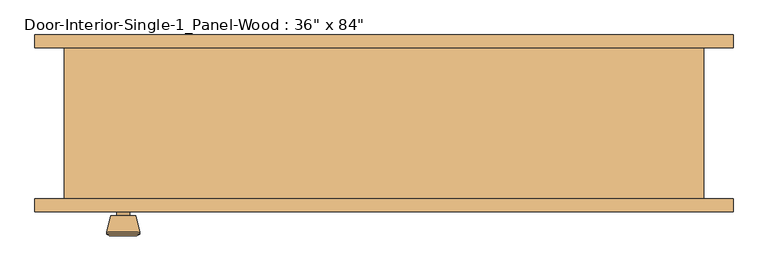
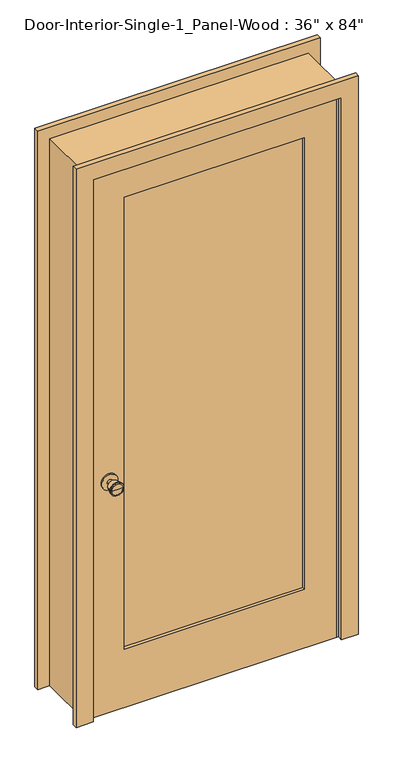
"""IFC4 building model written with IfcOpenShell, lengths in millimetres: door geometry."""

from ifc_helpers import new_model, si_unit, point, frame, frame_2d, origin, place, context, project, spatial, polyline, circle_curve, trimmed, segment, composite_curve, outline, extrude, faceted_brep, source, transform, mapped, element, save
from ifc_brep_helpers import plane_surface, cylinder_surface, revolved_surface, advanced_brep


def door_868ee8a9(model_context):
    return source(origin(), model_context, "Body", "SolidModel", [
        advanced_brep(
        [(-393.7, -70.2, 914.4), (-403.7, -70.2, 914.4), (-383.7, -70.2, 914.4), (-373.2241324, -21.2, 914.4), (-414.1758676, -21.2, 914.4), (-393.7, -21.2, 914.4), (-368.7, -23.0278681, 914.4), (-418.7, -23.0278681, 914.4), (-368.7, -26.4915463, 914.4), (-418.7, -26.4915463, 914.4), (-375.063764, -51.2, 914.4), (-412.336236, -51.2, 914.4), (-383.7, -51.2, 914.4), (-403.7, -51.2, 914.4)],
        [
            (0, 1),
            (1, 2, circle_curve(frame((-393.7, -70.2, 914.4), z_axis=(0.0, -1.0, 0.0), x_axis=(-1.0, 0.0, 0.0)), 10.0)),
            (2, 0),
            (2, 1, circle_curve(frame((-393.7, -70.2, 914.4), z_axis=(0.0, -1.0, 0.0), x_axis=(-1.0, 0.0, 0.0)), 10.0)),
            (3, 4, circle_curve(frame((-393.7, -21.2, 914.4), z_axis=(0.0, 1.0, 0.0), x_axis=(-1.0, 0.0, 0.0)), 20.4758676)),
            (4, 5),
            (5, 3),
            (4, 3, circle_curve(frame((-393.7, -21.2, 914.4), z_axis=(0.0, 1.0, 0.0), x_axis=(-1.0, 0.0, 0.0)), 20.4758676)),
            (6, 7, circle_curve(frame((-393.7, -23.0278681, 914.4), z_axis=(0.0, 1.0, 0.0), x_axis=(-1.0, 0.0, 0.0)), 25.0)),
            (7, 4),
            (3, 6),
            (7, 6, circle_curve(frame((-393.7, -23.0278681, 914.4), z_axis=(0.0, 1.0, 0.0), x_axis=(-1.0, 0.0, 0.0)), 25.0)),
            (8, 9, circle_curve(frame((-393.7, -26.4915463, 914.4), z_axis=(0.0, 1.0, 0.0), x_axis=(-1.0, 0.0, 0.0)), 25.0)),
            (9, 7),
            (6, 8),
            (9, 8, circle_curve(frame((-393.7, -26.4915463, 914.4), z_axis=(0.0, 1.0, 0.0), x_axis=(-1.0, 0.0, 0.0)), 25.0)),
            (10, 11, circle_curve(frame((-393.7, -51.2, 914.4), z_axis=(0.0, 1.0, 0.0), x_axis=(-1.0, 0.0, 0.0)), 18.636236)),
            (11, 9),
            (8, 10),
            (11, 10, circle_curve(frame((-393.7, -51.2, 914.4), z_axis=(0.0, 1.0, 0.0), x_axis=(-1.0, 0.0, 0.0)), 18.636236)),
            (12, 13, circle_curve(frame((-393.7, -51.2, 914.4), z_axis=(0.0, 1.0, 0.0), x_axis=(-1.0, 0.0, 0.0)), 10.0)),
            (13, 11),
            (10, 12),
            (13, 12, circle_curve(frame((-393.7, -51.2, 914.4), z_axis=(0.0, 1.0, 0.0), x_axis=(-1.0, 0.0, 0.0)), 10.0)),
            (1, 13),
            (12, 2),
        ],
        [
            plane_surface(frame((-393.7, -70.2, 914.4), z_axis=(0.0, -1.0, 0.0), x_axis=(-1.0, 0.0, 0.0))),
            plane_surface(frame((-393.7, -21.2, 914.4), z_axis=(0.0, 1.0, 0.0), x_axis=(-1.0, 0.0, 0.0))),
            revolved_surface(polyline([(-414.1758676, -21.2, 914.4), (-418.7, -23.0278681, 914.4)]), (-393.7, -70.2, 914.4), (0.0, -1.0, 0.0)),
            cylinder_surface(frame((-393.7, -70.2, 914.4), z_axis=(0.0, -1.0, 0.0), x_axis=(-1.0, 0.0, 0.0)), 25.0),
            revolved_surface(polyline([(-418.7, -26.4915463, 914.4), (-412.336236, -51.2, 914.4)]), (-393.7, -70.2, 914.4), (0.0, -1.0, 0.0)),
            plane_surface(frame((-393.7, -51.2, 914.4), z_axis=(0.0, -1.0, 0.0), x_axis=(-1.0, 0.0, 0.0))),
            cylinder_surface(frame((-393.7, -70.2, 914.4), z_axis=(0.0, -1.0, 0.0), x_axis=(-1.0, 0.0, 0.0)), 10.0),
        ],
        [
            (0, [[1, 2, 3]]),
            (0, [[-3, 4, -1]]),
            (1, [[5, 6, 7]]),
            (1, [[8, -7, -6]]),
            (2, [[9, 10, -5, 11]]),
            (2, [[12, -11, -8, -10]]),
            (3, [[13, 14, -9, 15]]),
            (3, [[16, -15, -12, -14]]),
            (4, [[17, 18, -13, 19]]),
            (4, [[20, -19, -16, -18]]),
            (5, [[21, 22, -17, 23]]),
            (5, [[24, -23, -20, -22]]),
            (6, [[-2, 25, -21, 26]]),
            (6, [[-4, -26, -24, -25]]),
        ],
    ),
        extrude(outline(composite_curve([segment(trimmed(circle_curve(frame_2d((914.4, -393.7)), 30.0), [point((914.4, -423.7))], [point((914.4, -363.7))], False, "CARTESIAN"), True, "CONTINUOUS"), segment(trimmed(circle_curve(frame_2d((914.4, -393.7)), 30.0), [point((914.4, -363.7))], [point((914.4, -423.7))], False, "CARTESIAN"), True, "CONTINUOUS")], self_intersect=False)), frame((0.0, -76.2, 0.0), z_axis=(0.0, 1.0, 0.0), x_axis=(0.0, 0.0, 1.0)), (0.0, 0.0, 1.0), 6.0),
        advanced_brep(
        [(-393.7, -117.125, 914.4), (-383.7, -117.125, 914.4), (-403.7, -117.125, 914.4), (-373.2241324, -166.125, 914.4), (-393.7, -166.125, 914.4), (-414.1758676, -166.125, 914.4), (-368.7, -164.2971319, 914.4), (-418.7, -164.2971319, 914.4), (-368.7, -160.8334537, 914.4), (-418.7, -160.8334537, 914.4), (-375.063764, -136.125, 914.4), (-412.336236, -136.125, 914.4), (-383.7, -136.125, 914.4), (-403.7, -136.125, 914.4)],
        [
            (0, 1),
            (1, 2, circle_curve(frame((-393.7, -117.125, 914.4), z_axis=(0.0, 1.0, 0.0), x_axis=(-1.0, 0.0, 0.0)), 10.0)),
            (2, 0),
            (2, 1, circle_curve(frame((-393.7, -117.125, 914.4), z_axis=(0.0, 1.0, 0.0), x_axis=(-1.0, 0.0, 0.0)), 10.0)),
            (3, 4),
            (4, 5),
            (5, 3, circle_curve(frame((-393.7, -166.125, 914.4), z_axis=(0.0, -1.0, 0.0), x_axis=(-1.0, 0.0, 0.0)), 20.4758676)),
            (3, 5, circle_curve(frame((-393.7, -166.125, 914.4), z_axis=(0.0, -1.0, 0.0), x_axis=(-1.0, 0.0, 0.0)), 20.4758676)),
            (6, 3),
            (5, 7),
            (7, 6, circle_curve(frame((-393.7, -164.2971319, 914.4), z_axis=(0.0, -1.0, 0.0), x_axis=(-1.0, 0.0, 0.0)), 25.0)),
            (6, 7, circle_curve(frame((-393.7, -164.2971319, 914.4), z_axis=(0.0, -1.0, 0.0), x_axis=(-1.0, 0.0, 0.0)), 25.0)),
            (8, 6),
            (7, 9),
            (9, 8, circle_curve(frame((-393.7, -160.8334537, 914.4), z_axis=(0.0, -1.0, 0.0), x_axis=(-1.0, 0.0, 0.0)), 25.0)),
            (8, 9, circle_curve(frame((-393.7, -160.8334537, 914.4), z_axis=(0.0, -1.0, 0.0), x_axis=(-1.0, 0.0, 0.0)), 25.0)),
            (10, 8),
            (9, 11),
            (11, 10, circle_curve(frame((-393.7, -136.125, 914.4), z_axis=(0.0, -1.0, 0.0), x_axis=(-1.0, 0.0, 0.0)), 18.636236)),
            (10, 11, circle_curve(frame((-393.7, -136.125, 914.4), z_axis=(0.0, -1.0, 0.0), x_axis=(-1.0, 0.0, 0.0)), 18.636236)),
            (12, 10),
            (11, 13),
            (13, 12, circle_curve(frame((-393.7, -136.125, 914.4), z_axis=(0.0, -1.0, 0.0), x_axis=(-1.0, 0.0, 0.0)), 10.0)),
            (12, 13, circle_curve(frame((-393.7, -136.125, 914.4), z_axis=(0.0, -1.0, 0.0), x_axis=(-1.0, 0.0, 0.0)), 10.0)),
            (1, 12),
            (13, 2),
        ],
        [
            plane_surface(frame((-393.7, -117.125, 914.4), z_axis=(0.0, 1.0, 0.0), x_axis=(-1.0, 0.0, 0.0))),
            plane_surface(frame((-393.7, -166.125, 914.4), z_axis=(0.0, -1.0, 0.0), x_axis=(-1.0, 0.0, 0.0))),
            revolved_surface(polyline([(-414.1758676, -166.125, 914.4), (-418.7, -164.2971319, 914.4)]), (-393.7, -117.125, 914.4), (0.0, 1.0, 0.0)),
            cylinder_surface(frame((-393.7, -117.125, 914.4), z_axis=(0.0, 1.0, 0.0), x_axis=(-1.0, 0.0, 0.0)), 25.0),
            revolved_surface(polyline([(-418.7, -160.8334537, 914.4), (-412.336236, -136.125, 914.4)]), (-393.7, -117.125, 914.4), (0.0, 1.0, 0.0)),
            plane_surface(frame((-393.7, -136.125, 914.4), z_axis=(0.0, 1.0, 0.0), x_axis=(-1.0, 0.0, 0.0))),
            cylinder_surface(frame((-393.7, -117.125, 914.4), z_axis=(0.0, 1.0, 0.0), x_axis=(-1.0, 0.0, 0.0)), 10.0),
        ],
        [
            (0, [[1, 2, 3]]),
            (0, [[-3, 4, -1]]),
            (1, [[5, 6, 7]]),
            (1, [[-6, -5, 8]]),
            (2, [[9, -7, 10, 11]]),
            (2, [[-10, -8, -9, 12]]),
            (3, [[13, -11, 14, 15]]),
            (3, [[-14, -12, -13, 16]]),
            (4, [[17, -15, 18, 19]]),
            (4, [[-18, -16, -17, 20]]),
            (5, [[21, -19, 22, 23]]),
            (5, [[-22, -20, -21, 24]]),
            (6, [[25, -23, 26, -2]]),
            (6, [[-26, -24, -25, -4]]),
        ],
    ),
        extrude(outline(composite_curve([segment(trimmed(circle_curve(frame_2d((914.4, -393.7)), 30.0), [point((914.4, -423.7))], [point((914.4, -363.7))], False, "CARTESIAN"), True, "CONTINUOUS"), segment(trimmed(circle_curve(frame_2d((914.4, -393.7)), 30.0), [point((914.4, -363.7))], [point((914.4, -423.7))], False, "CARTESIAN"), True, "CONTINUOUS")], self_intersect=False)), frame((0.0, -117.125, 0.0), z_axis=(0.0, 1.0, 0.0), x_axis=(0.0, 0.0, 1.0)), (0.0, 0.0, 1.0), 6.0),
        faceted_brep([(482.6, -111.125, 0.0), (457.2, -111.125, 0.0), (457.2, -76.2, 0.0), (444.5, -76.2, 0.0), (444.5, -41.275, 0.0), (457.2, -41.275, 0.0), (457.2, 117.475, 0.0), (482.6, 117.475, 0.0), (482.6, 117.475, 2159.0), (482.6, -111.125, 2159.0), (457.2, 117.475, 2133.6), (-457.2, 117.475, 2133.6), (-457.2, 117.475, 0.0), (-482.6, 117.475, 0.0), (-482.6, 117.475, 2159.0), (457.2, -41.275, 2133.6), (444.5, -41.275, 2120.9), (-444.5, -41.275, 2120.9), (-444.5, -41.275, 0.0), (-457.2, -41.275, 0.0), (-457.2, -41.275, 2133.6), (444.5, -76.2, 2120.9), (457.2, -76.2, 2133.6), (-457.2, -76.2, 2133.6), (-457.2, -76.2, 0.0), (-444.5, -76.2, 0.0), (-444.5, -76.2, 2120.9), (457.2, -111.125, 2133.6), (-482.6, -111.125, 2159.0), (-482.6, -111.125, 0.0), (-457.2, -111.125, 0.0), (-457.2, -111.125, 2133.6)], [[[0, 1, 2, 3, 4, 5, 6, 7]], [[7, 8, 9, 0]], [[6, 10, 11, 12, 13, 14, 8, 7]], [[5, 15, 10, 6]], [[4, 16, 17, 18, 19, 20, 15, 5]], [[3, 21, 16, 4]], [[2, 22, 23, 24, 25, 26, 21, 3]], [[1, 27, 22, 2]], [[0, 9, 28, 29, 30, 31, 27, 1]], [[8, 14, 28, 9]], [[15, 20, 11, 10]], [[21, 26, 17, 16]], [[27, 31, 23, 22]], [[29, 13, 12, 19, 18, 25, 24, 30]], [[14, 13, 29, 28]], [[20, 19, 12, 11]], [[26, 25, 18, 17]], [[31, 30, 24, 23]]]),
        extrude(outline(polyline([(2133.6, -457.2), (0.0, -457.2), (0.0, 457.2), (2133.6, 457.2), (2133.6, -457.2)]), holes=[polyline([(2014.5375, -336.55), (2014.5375, 336.55), (231.775, 336.55), (231.775, -336.55), (2014.5375, -336.55)])]), frame((0.0, -111.125, 0.0), z_axis=(0.0, 1.0, 0.0), x_axis=(0.0, 0.0, 1.0)), (0.0, 0.0, 1.0), 34.925),
        extrude(outline(polyline([(336.55, -87.8416667), (336.55, -99.4833333), (-336.55, -99.4833333), (-336.55, -87.8416667), (336.55, -87.8416667)])), frame((0.0, 0.0, 231.775), z_axis=(0.0, 0.0, 1.0), x_axis=(1.0, 0.0, 0.0)), (0.0, 0.0, 1.0), 1782.7625),
        extrude(outline(polyline([(0.0, 527.05), (2203.45, 527.05), (2203.45, -527.05), (0.0, -527.05), (0.0, -463.55), (2139.95, -463.55), (2139.95, 463.55), (0.0, 463.55), (0.0, 527.05)])), frame((0.0, -130.175, 0.0), z_axis=(0.0, 1.0, 0.0), x_axis=(0.0, 0.0, 1.0)), (0.0, 0.0, 1.0), 19.05),
        extrude(outline(polyline([(0.0, 527.05), (2203.45, 527.05), (2203.45, -527.05), (0.0, -527.05), (0.0, -463.55), (2139.95, -463.55), (2139.95, 463.55), (0.0, 463.55), (0.0, 527.05)])), frame((0.0, 117.475, 0.0), z_axis=(0.0, 1.0, 0.0), x_axis=(0.0, 0.0, 1.0)), (0.0, 0.0, 1.0), 19.05),
    ])


if __name__ == "__main__":
    model = new_model("IFC4")
    model_context = context("Model", 3, world=origin())
    ifc_project = project(units=[si_unit("LENGTHUNIT", "METRE", prefix="MILLI")], contexts=[model_context])
    site = spatial("IfcSite", under=ifc_project)
    building = spatial("IfcBuilding", under=site)
    placement = place(None, origin())
    door_shape = door_868ee8a9(model_context)
    element("IfcDoor", 1, ObjectType="Door-Interior-Single-1_Panel-Wood : 36\" x 84\"", at=placement, inside=building, context=model_context, shape_type="MappedRepresentation", body=[
        mapped(door_shape, transform((0.0, 0.0, 0.0), x_axis=(1.0, 0.0, 0.0), y_axis=(0.0, 1.0, 0.0), z_axis=(0.0, 0.0, 1.0))),
    ])
    save(model, "model.ifc")

# Revit data of these elements
# Type "Door-Interior-Single-1_Panel-Wood : 36\" x 84\""
#   Type Mark = "17"
#   Assembly Code = "C1020300"
#   Analytic Construction = "Wooden"
#   Top Rail = 0' - 4 11/16"
#   Thickness = 0' - 1 3/8"
#   Thermal Resistance (R) = 2.5876 (h·ft²·°F)/BTU
#   Swing Angle [instance default] = 90.00°
#   Stiles = 0' - 4 3/4"
#   Rough Width = 3' - 2"
#   Rough Height = 7' - 1"
#   Height = 7' - 0"
#   Width = 3' - 0"
#   Heat Transfer Coefficient (U) = 0.3865 BTU/(h·ft²·°F)
#   Bottom Rail = 0' - 9 1/8"
#   Trim Material = Cherry
#   Panel Material = Cherry
#   Frame Material = Cherry
#   Door Handle Material = Aluminum
#   Visual Light Transmittance = 0
#   Solar Heat Gain Coefficient = 0
#   Wall Closure = (empty or 0)
#   Function = (empty or 0)
# Element 1 (IfcDoor, "Door-Interior-Single-1_Panel-Wood : 36\" x 84\"")
#   Materials on its faces: "Cherry", "Aluminum"
# Materials
#   "Cherry": class "Wood", colour RGB 226 177 128, transparency 0, Description = "Prunus Serotina", Cost = 0
#   "Aluminum": class "Metal", colour RGB 247 247 247, transparency 0, Description = "Aluminum 6061", Cost = 0
